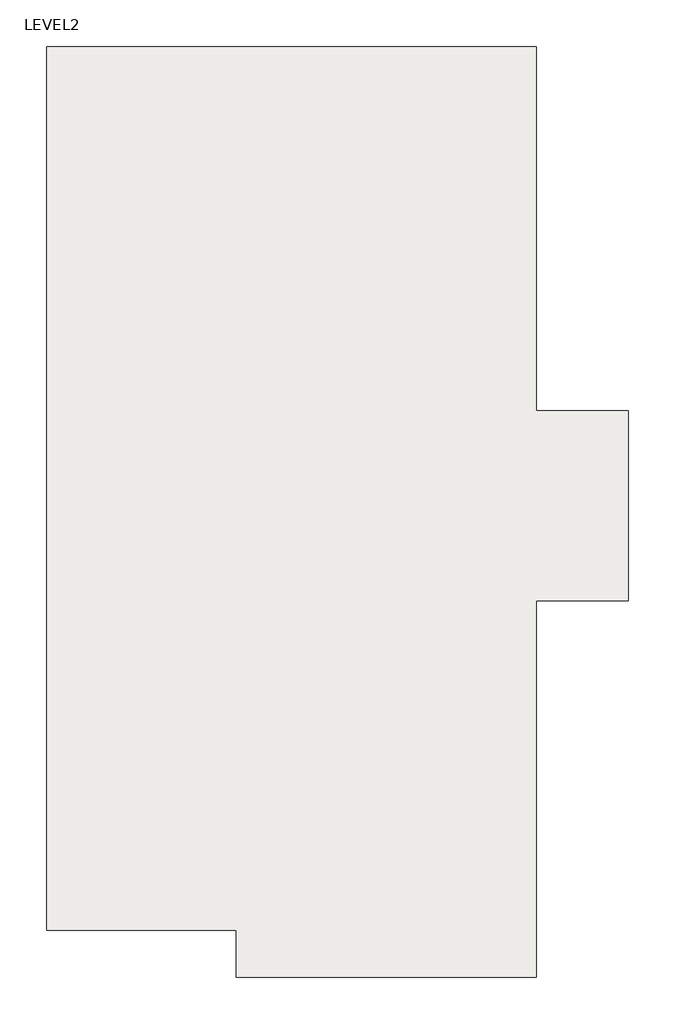
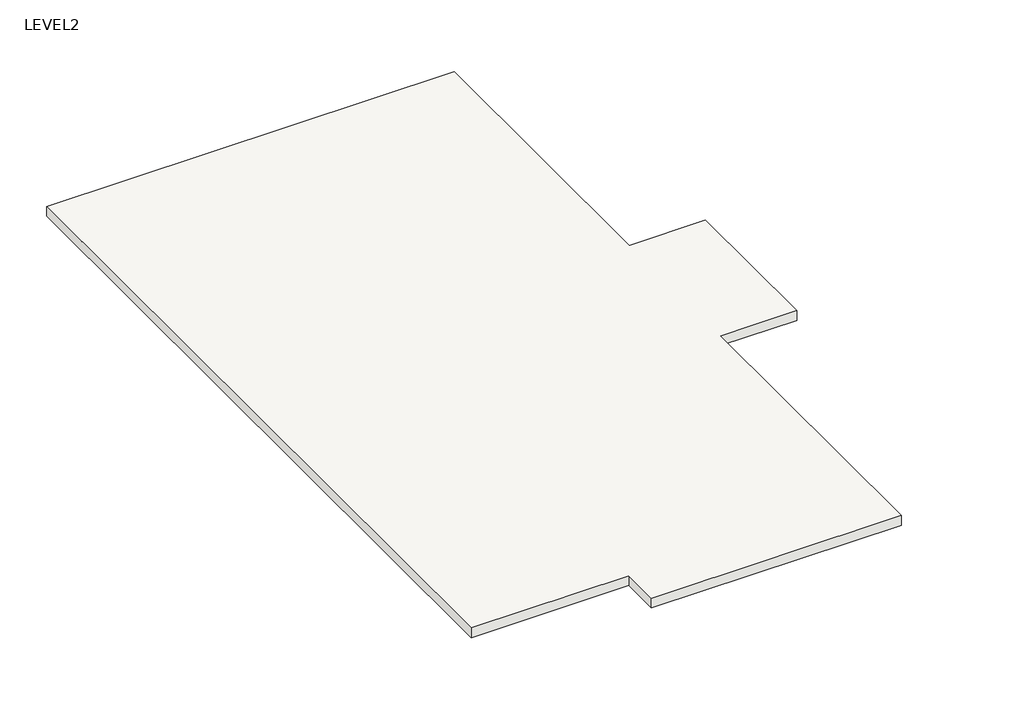
# One storey, incomplete: 1 roof.
"""IFC4 building model written with IfcOpenShell, lengths in millimetres."""

from ifc_helpers import new_model, si_unit, frame, origin, place, context, project, spatial, polyline, outline, extrude, element, save

model = new_model("IFC4")

# Units and contexts
model_context = context("Model", 3, world=origin())
ifc_project = project(units=[si_unit("LENGTHUNIT", "METRE", prefix="MILLI")], contexts=[model_context])

# Site, building, storey
site = spatial("IfcSite", under=ifc_project)
building = spatial("IfcBuilding", under=site)
storey = spatial("IfcBuildingStorey", under=building, Name="LEVEL2", Elevation=3048.0)

# Roof
placement = place(None, origin())
element("IfcRoof", 1, ObjectType="Generic - 12\"", at=placement, inside=storey, context=model_context, shape_type="SweptSolid", body=[
    extrude(outline(polyline([(1270.0, 14224.0), (7366.0, 14224.0), (7366.0, 9690.1), (8509.0, 9690.1), (8509.0, 7327.9), (7366.0, 7327.9), (7366.0, 2641.6), (3632.2, 2641.6), (3632.2, 3225.8), (1270.0, 3225.8), (1270.0, 14224.0)])), frame((0.0, 0.0, 3048.0), z_axis=(0.0, 0.0, 1.0), x_axis=(1.0, 0.0, 0.0)), (0.0, 0.0, 1.0), 152.4),
])

save(model, "model.ifc")

# Revit data of these elements
# Type "Generic - 12\""
#   Assembly Code = "B1020"
#   Layers, outside or top first: 0' - 6" no material (function 1)
# Element 1 (IfcRoof, "Generic - 12\"")
#   built-in parameter 1001705 = 10.5 (stored number, unit not read)
#   built-in parameter 1001710 = 33615
#   Phase Created = New Construction
#   Materials on its faces: "Clad - White", "Default Roof"
# Materials
#   "Clad - White": class "Wood", colour RGB 242 242 238, transparency 0, Cost = 0
#   "Default Roof": colour RGB 88 101 114, transparency 0, Cost = 0
